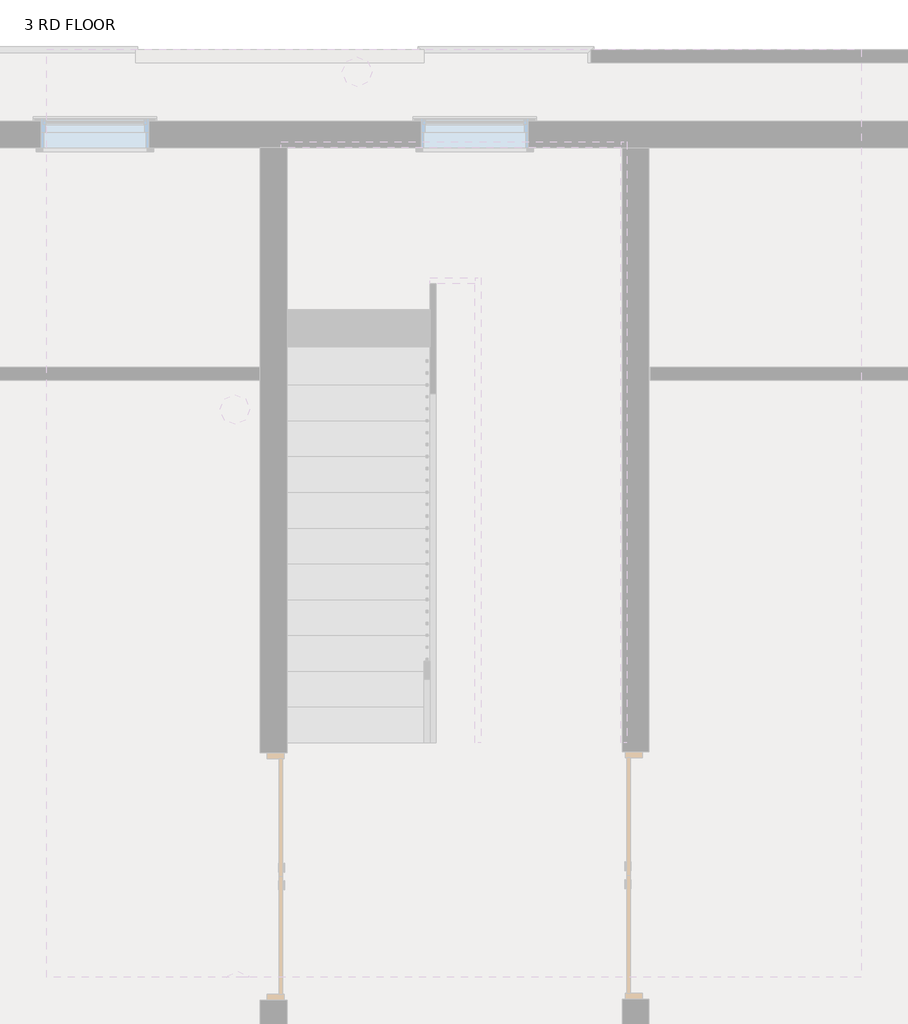
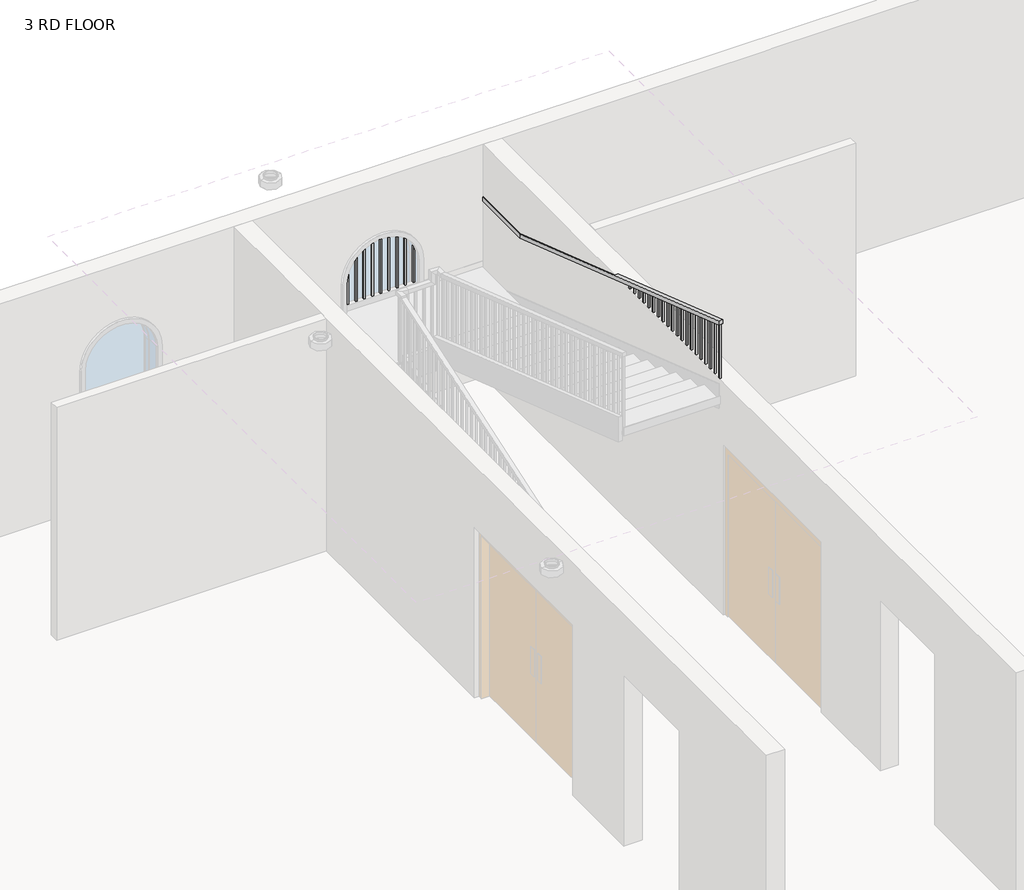
# One storey, part 5 of 7: 1 railing.
"""IFC4 building model written with IfcOpenShell, lengths in millimetres."""

from ifc_helpers import new_model, si_unit, frame, origin, place, context, project, spatial, polyline, outline, extrude, faceted_brep, element, save

model = new_model("IFC4")

# Units and contexts
model_context = context("Model", 3, world=origin())
ifc_project = project(units=[si_unit("LENGTHUNIT", "METRE", prefix="MILLI")], contexts=[model_context])

# Site, building, storey
site = spatial("IfcSite", under=ifc_project)
building = spatial("IfcBuilding", under=site)
storey = spatial("IfcBuildingStorey", under=building, Name="3 RD FLOOR", Elevation=9601.2)

# Railing
placement = place(None, origin())
element("IfcRailing", 1, ObjectType="Handrail - Rectangular", at=placement, inside=storey, context=model_context, shape_type="SolidModel", body=[
    faceted_brep([(-1899.5987998, 2564.5067329, 10619.0142857), (-1899.5987998, 2564.5067329, 10565.3699957), (-1848.7987998, 2564.5067329, 10565.3699957), (-1848.7987998, 2564.5067329, 10619.0142857), (-1899.5987998, 6526.9067329, 11963.4), (-1899.5987998, 6535.2899033, 11912.6), (-1848.7987998, 6535.2899033, 11912.6), (-1848.7987998, 6526.9067329, 11963.4), (-1899.5987998, 7682.6067329, 11912.6), (-1899.5987998, 7682.6067329, 11963.4), (1046.8012002, 7682.6067329, 11963.4), (1046.8012002, 7682.6067329, 11912.6), (-1848.7987998, 7631.8067329, 11912.6), (996.0012002, 7631.8067329, 11912.6), (-1848.7987998, 7631.8067329, 11963.4), (996.0012002, 7631.8067329, 11963.4), (1046.8012002, 6831.7067329, 11963.4), (1046.8012002, 6823.3235624, 11912.6), (996.0012002, 6823.3235624, 11912.6), (996.0012002, 6831.7067329, 11963.4), (1046.8012002, 2564.5067329, 13411.2), (996.0012002, 2564.5067329, 13411.2), (996.0012002, 2564.5067329, 13357.55571), (1046.8012002, 2564.5067329, 13357.55571)], [[[0, 1, 2, 3]], [[1, 0, 4, 5]], [[2, 1, 5, 6]], [[3, 2, 6, 7]], [[0, 3, 7, 4]], [[8, 9, 10, 11]], [[12, 8, 11, 13]], [[14, 12, 13, 15]], [[9, 14, 15, 10]], [[11, 10, 16, 17]], [[13, 11, 17, 18]], [[15, 13, 18, 19]], [[10, 15, 19, 16]], [[5, 4, 9, 8]], [[6, 5, 8, 12]], [[7, 6, 12, 14]], [[4, 7, 14, 9]], [[20, 21, 22, 23]], [[17, 16, 20, 23]], [[18, 17, 23, 22]], [[19, 18, 22, 21]], [[16, 19, 21, 20]]]),
    extrude(outline(polyline([(2586.7317329, 13350.015085), (2586.7317329, 12579.0831452), (2567.6817329, 12585.5465381), (2567.6817329, 13356.4784779), (2586.7317329, 13350.015085)])), frame((1011.8762002, 0.0, 0.0), z_axis=(1.0, 0.0, 0.0), x_axis=(0.0, 1.0, 0.0)), (0.0, 0.0, 1.0), 19.05),
    extrude(outline(polyline([(2688.3317329, 13315.5436565), (2688.3317329, 12544.6117167), (2669.2817329, 12551.0751095), (2669.2817329, 13322.0070493), (2688.3317329, 13315.5436565)])), frame((1011.8762002, 0.0, 0.0), z_axis=(1.0, 0.0, 0.0), x_axis=(0.0, 1.0, 0.0)), (0.0, 0.0, 1.0), 19.05),
    extrude(outline(polyline([(2789.9317329, 13281.0722279), (2789.9317329, 12510.1402881), (2770.8817329, 12516.603681), (2770.8817329, 13287.5356207), (2789.9317329, 13281.0722279)])), frame((1011.8762002, 0.0, 0.0), z_axis=(1.0, 0.0, 0.0), x_axis=(0.0, 1.0, 0.0)), (0.0, 0.0, 1.0), 19.05),
    extrude(outline(polyline([(2891.5317329, 13246.6007993), (2891.5317329, 12475.6688595), (2872.4817329, 12482.1322524), (2872.4817329, 13253.0641922), (2891.5317329, 13246.6007993)])), frame((1011.8762002, 0.0, 0.0), z_axis=(1.0, 0.0, 0.0), x_axis=(0.0, 1.0, 0.0)), (0.0, 0.0, 1.0), 19.05),
    extrude(outline(polyline([(2993.1317329, 13212.1293707), (2993.1317329, 12441.197431), (2974.0817329, 12447.6608238), (2974.0817329, 13218.5927636), (2993.1317329, 13212.1293707)])), frame((1011.8762002, 0.0, 0.0), z_axis=(1.0, 0.0, 0.0), x_axis=(0.0, 1.0, 0.0)), (0.0, 0.0, 1.0), 19.05),
    extrude(outline(polyline([(3094.7317329, 13177.6579422), (3094.7317329, 12406.7260024), (3075.6817329, 12413.1893952), (3075.6817329, 13184.121335), (3094.7317329, 13177.6579422)])), frame((1011.8762002, 0.0, 0.0), z_axis=(1.0, 0.0, 0.0), x_axis=(0.0, 1.0, 0.0)), (0.0, 0.0, 1.0), 19.05),
    extrude(outline(polyline([(3196.3317329, 13143.1865136), (3196.3317329, 12372.2545738), (3177.2817329, 12378.7179667), (3177.2817329, 13149.6499065), (3196.3317329, 13143.1865136)])), frame((1011.8762002, 0.0, 0.0), z_axis=(1.0, 0.0, 0.0), x_axis=(0.0, 1.0, 0.0)), (0.0, 0.0, 1.0), 19.05),
    extrude(outline(polyline([(3297.9317329, 13108.715085), (3297.9317329, 12337.7831452), (3278.8817329, 12344.2465381), (3278.8817329, 13115.1784779), (3297.9317329, 13108.715085)])), frame((1011.8762002, 0.0, 0.0), z_axis=(1.0, 0.0, 0.0), x_axis=(0.0, 1.0, 0.0)), (0.0, 0.0, 1.0), 19.05),
    extrude(outline(polyline([(3399.5317329, 13074.2436565), (3399.5317329, 12303.3117167), (3380.4817329, 12309.7751095), (3380.4817329, 13080.7070493), (3399.5317329, 13074.2436565)])), frame((1011.8762002, 0.0, 0.0), z_axis=(1.0, 0.0, 0.0), x_axis=(0.0, 1.0, 0.0)), (0.0, 0.0, 1.0), 19.05),
    extrude(outline(polyline([(3501.1317329, 13039.7722279), (3501.1317329, 12268.8402881), (3482.0817329, 12275.303681), (3482.0817329, 13046.2356207), (3501.1317329, 13039.7722279)])), frame((1011.8762002, 0.0, 0.0), z_axis=(1.0, 0.0, 0.0), x_axis=(0.0, 1.0, 0.0)), (0.0, 0.0, 1.0), 19.05),
    extrude(outline(polyline([(3602.7317329, 13005.3007993), (3602.7317329, 12234.3688595), (3583.6817329, 12240.8322524), (3583.6817329, 13011.7641922), (3602.7317329, 13005.3007993)])), frame((1011.8762002, 0.0, 0.0), z_axis=(1.0, 0.0, 0.0), x_axis=(0.0, 1.0, 0.0)), (0.0, 0.0, 1.0), 19.05),
    extrude(outline(polyline([(3704.3317329, 12970.8293707), (3704.3317329, 12199.897431), (3685.2817329, 12206.3608238), (3685.2817329, 12977.2927636), (3704.3317329, 12970.8293707)])), frame((1011.8762002, 0.0, 0.0), z_axis=(1.0, 0.0, 0.0), x_axis=(0.0, 1.0, 0.0)), (0.0, 0.0, 1.0), 19.05),
    extrude(outline(polyline([(3805.9317329, 12936.3579422), (3805.9317329, 12165.4260024), (3786.8817329, 12171.8893952), (3786.8817329, 12942.821335), (3805.9317329, 12936.3579422)])), frame((1011.8762002, 0.0, 0.0), z_axis=(1.0, 0.0, 0.0), x_axis=(0.0, 1.0, 0.0)), (0.0, 0.0, 1.0), 19.05),
    extrude(outline(polyline([(3907.5317329, 12901.8865136), (3907.5317329, 12130.9545738), (3888.4817329, 12137.4179667), (3888.4817329, 12908.3499065), (3907.5317329, 12901.8865136)])), frame((1011.8762002, 0.0, 0.0), z_axis=(1.0, 0.0, 0.0), x_axis=(0.0, 1.0, 0.0)), (0.0, 0.0, 1.0), 19.05),
    extrude(outline(polyline([(4009.1317329, 12867.415085), (4009.1317329, 12096.4831452), (3990.0817329, 12102.9465381), (3990.0817329, 12873.8784779), (4009.1317329, 12867.415085)])), frame((1011.8762002, 0.0, 0.0), z_axis=(1.0, 0.0, 0.0), x_axis=(0.0, 1.0, 0.0)), (0.0, 0.0, 1.0), 19.05),
    extrude(outline(polyline([(4110.7317329, 12832.9436565), (4110.7317329, 12062.0117167), (4091.6817329, 12068.4751095), (4091.6817329, 12839.4070493), (4110.7317329, 12832.9436565)])), frame((1011.8762002, 0.0, 0.0), z_axis=(1.0, 0.0, 0.0), x_axis=(0.0, 1.0, 0.0)), (0.0, 0.0, 1.0), 19.05),
    extrude(outline(polyline([(4212.3317329, 12798.4722279), (4212.3317329, 12027.5402881), (4193.2817329, 12034.003681), (4193.2817329, 12804.9356207), (4212.3317329, 12798.4722279)])), frame((1011.8762002, 0.0, 0.0), z_axis=(1.0, 0.0, 0.0), x_axis=(0.0, 1.0, 0.0)), (0.0, 0.0, 1.0), 19.05),
    extrude(outline(polyline([(4313.9317329, 12764.0007993), (4313.9317329, 11993.0688595), (4294.8817329, 11999.5322524), (4294.8817329, 12770.4641922), (4313.9317329, 12764.0007993)])), frame((1011.8762002, 0.0, 0.0), z_axis=(1.0, 0.0, 0.0), x_axis=(0.0, 1.0, 0.0)), (0.0, 0.0, 1.0), 19.05),
    extrude(outline(polyline([(4415.5317329, 12729.5293707), (4415.5317329, 11958.597431), (4396.4817329, 11965.0608238), (4396.4817329, 12735.9927636), (4415.5317329, 12729.5293707)])), frame((1011.8762002, 0.0, 0.0), z_axis=(1.0, 0.0, 0.0), x_axis=(0.0, 1.0, 0.0)), (0.0, 0.0, 1.0), 19.05),
    extrude(outline(polyline([(4517.1317329, 12695.0579422), (4517.1317329, 11924.1260024), (4498.0817329, 11930.5893952), (4498.0817329, 12701.521335), (4517.1317329, 12695.0579422)])), frame((1011.8762002, 0.0, 0.0), z_axis=(1.0, 0.0, 0.0), x_axis=(0.0, 1.0, 0.0)), (0.0, 0.0, 1.0), 19.05),
    extrude(outline(polyline([(4618.7317329, 12660.5865136), (4618.7317329, 11889.6545738), (4599.6817329, 11896.1179667), (4599.6817329, 12667.0499065), (4618.7317329, 12660.5865136)])), frame((1011.8762002, 0.0, 0.0), z_axis=(1.0, 0.0, 0.0), x_axis=(0.0, 1.0, 0.0)), (0.0, 0.0, 1.0), 19.05),
    extrude(outline(polyline([(4720.3317329, 12626.115085), (4720.3317329, 11855.1831452), (4701.2817329, 11861.6465381), (4701.2817329, 12632.5784779), (4720.3317329, 12626.115085)])), frame((1011.8762002, 0.0, 0.0), z_axis=(1.0, 0.0, 0.0), x_axis=(0.0, 1.0, 0.0)), (0.0, 0.0, 1.0), 19.05),
    extrude(outline(polyline([(4821.9317329, 12591.6436565), (4821.9317329, 11820.7117167), (4802.8817329, 11827.1751095), (4802.8817329, 12598.1070493), (4821.9317329, 12591.6436565)])), frame((1011.8762002, 0.0, 0.0), z_axis=(1.0, 0.0, 0.0), x_axis=(0.0, 1.0, 0.0)), (0.0, 0.0, 1.0), 19.05),
    extrude(outline(polyline([(4923.5317329, 12557.1722279), (4923.5317329, 11786.2402881), (4904.4817329, 11792.703681), (4904.4817329, 12563.6356207), (4923.5317329, 12557.1722279)])), frame((1011.8762002, 0.0, 0.0), z_axis=(1.0, 0.0, 0.0), x_axis=(0.0, 1.0, 0.0)), (0.0, 0.0, 1.0), 19.05),
    extrude(outline(polyline([(5025.1317329, 12522.7007993), (5025.1317329, 11751.7688595), (5006.0817329, 11758.2322524), (5006.0817329, 12529.1641922), (5025.1317329, 12522.7007993)])), frame((1011.8762002, 0.0, 0.0), z_axis=(1.0, 0.0, 0.0), x_axis=(0.0, 1.0, 0.0)), (0.0, 0.0, 1.0), 19.05),
    extrude(outline(polyline([(5126.7317329, 12488.2293707), (5126.7317329, 11717.297431), (5107.6817329, 11723.7608238), (5107.6817329, 12494.6927636), (5126.7317329, 12488.2293707)])), frame((1011.8762002, 0.0, 0.0), z_axis=(1.0, 0.0, 0.0), x_axis=(0.0, 1.0, 0.0)), (0.0, 0.0, 1.0), 19.05),
    extrude(outline(polyline([(5228.3317329, 12453.7579422), (5228.3317329, 11682.8260024), (5209.2817329, 11689.2893952), (5209.2817329, 12460.221335), (5228.3317329, 12453.7579422)])), frame((1011.8762002, 0.0, 0.0), z_axis=(1.0, 0.0, 0.0), x_axis=(0.0, 1.0, 0.0)), (0.0, 0.0, 1.0), 19.05),
    extrude(outline(polyline([(5329.9317329, 12419.2865136), (5329.9317329, 11648.3545738), (5310.8817329, 11654.8179667), (5310.8817329, 12425.7499065), (5329.9317329, 12419.2865136)])), frame((1011.8762002, 0.0, 0.0), z_axis=(1.0, 0.0, 0.0), x_axis=(0.0, 1.0, 0.0)), (0.0, 0.0, 1.0), 19.05),
    extrude(outline(polyline([(5431.5317329, 12384.815085), (5431.5317329, 11613.8831452), (5412.4817329, 11620.3465381), (5412.4817329, 12391.2784779), (5431.5317329, 12384.815085)])), frame((1011.8762002, 0.0, 0.0), z_axis=(1.0, 0.0, 0.0), x_axis=(0.0, 1.0, 0.0)), (0.0, 0.0, 1.0), 19.05),
    extrude(outline(polyline([(5533.1317329, 12350.3436565), (5533.1317329, 11579.4117167), (5514.0817329, 11585.8751095), (5514.0817329, 12356.8070493), (5533.1317329, 12350.3436565)])), frame((1011.8762002, 0.0, 0.0), z_axis=(1.0, 0.0, 0.0), x_axis=(0.0, 1.0, 0.0)), (0.0, 0.0, 1.0), 19.05),
    extrude(outline(polyline([(5634.7317329, 12315.8722279), (5634.7317329, 11544.9402881), (5615.6817329, 11551.403681), (5615.6817329, 12322.3356207), (5634.7317329, 12315.8722279)])), frame((1011.8762002, 0.0, 0.0), z_axis=(1.0, 0.0, 0.0), x_axis=(0.0, 1.0, 0.0)), (0.0, 0.0, 1.0), 19.05),
    extrude(outline(polyline([(5736.3317329, 12281.4007993), (5736.3317329, 11510.4688595), (5717.2817329, 11516.9322524), (5717.2817329, 12287.8641922), (5736.3317329, 12281.4007993)])), frame((1011.8762002, 0.0, 0.0), z_axis=(1.0, 0.0, 0.0), x_axis=(0.0, 1.0, 0.0)), (0.0, 0.0, 1.0), 19.05),
    extrude(outline(polyline([(5837.9317329, 12246.9293707), (5837.9317329, 11475.997431), (5818.8817329, 11482.4608238), (5818.8817329, 12253.3927636), (5837.9317329, 12246.9293707)])), frame((1011.8762002, 0.0, 0.0), z_axis=(1.0, 0.0, 0.0), x_axis=(0.0, 1.0, 0.0)), (0.0, 0.0, 1.0), 19.05),
    extrude(outline(polyline([(5939.5317329, 12212.4579422), (5939.5317329, 11441.5260024), (5920.4817329, 11447.9893952), (5920.4817329, 12218.921335), (5939.5317329, 12212.4579422)])), frame((1011.8762002, 0.0, 0.0), z_axis=(1.0, 0.0, 0.0), x_axis=(0.0, 1.0, 0.0)), (0.0, 0.0, 1.0), 19.05),
    extrude(outline(polyline([(6041.1317329, 12177.9865136), (6041.1317329, 11407.0545738), (6022.0817329, 11413.5179667), (6022.0817329, 12184.4499065), (6041.1317329, 12177.9865136)])), frame((1011.8762002, 0.0, 0.0), z_axis=(1.0, 0.0, 0.0), x_axis=(0.0, 1.0, 0.0)), (0.0, 0.0, 1.0), 19.05),
    extrude(outline(polyline([(6142.7317329, 12143.515085), (6142.7317329, 11372.5831452), (6123.6817329, 11379.0465381), (6123.6817329, 12149.9784779), (6142.7317329, 12143.515085)])), frame((1011.8762002, 0.0, 0.0), z_axis=(1.0, 0.0, 0.0), x_axis=(0.0, 1.0, 0.0)), (0.0, 0.0, 1.0), 19.05),
    extrude(outline(polyline([(6244.3317329, 12109.0436565), (6244.3317329, 11338.1117167), (6225.2817329, 11344.5751095), (6225.2817329, 12115.5070493), (6244.3317329, 12109.0436565)])), frame((1011.8762002, 0.0, 0.0), z_axis=(1.0, 0.0, 0.0), x_axis=(0.0, 1.0, 0.0)), (0.0, 0.0, 1.0), 19.05),
    extrude(outline(polyline([(6345.9317329, 12074.5722279), (6345.9317329, 11303.6402881), (6326.8817329, 11310.103681), (6326.8817329, 12081.0356207), (6345.9317329, 12074.5722279)])), frame((1011.8762002, 0.0, 0.0), z_axis=(1.0, 0.0, 0.0), x_axis=(0.0, 1.0, 0.0)), (0.0, 0.0, 1.0), 19.05),
    extrude(outline(polyline([(6447.5317329, 12040.1007993), (6447.5317329, 11269.1688595), (6428.4817329, 11275.6322524), (6428.4817329, 12046.5641922), (6447.5317329, 12040.1007993)])), frame((1011.8762002, 0.0, 0.0), z_axis=(1.0, 0.0, 0.0), x_axis=(0.0, 1.0, 0.0)), (0.0, 0.0, 1.0), 19.05),
    extrude(outline(polyline([(6549.1317329, 12005.6293707), (6549.1317329, 11234.697431), (6530.0817329, 11241.1608238), (6530.0817329, 12012.0927636), (6549.1317329, 12005.6293707)])), frame((1011.8762002, 0.0, 0.0), z_axis=(1.0, 0.0, 0.0), x_axis=(0.0, 1.0, 0.0)), (0.0, 0.0, 1.0), 19.05),
    extrude(outline(polyline([(6650.7317329, 11971.1579422), (6650.7317329, 11200.2260024), (6631.6817329, 11206.6893952), (6631.6817329, 11977.621335), (6650.7317329, 11971.1579422)])), frame((1011.8762002, 0.0, 0.0), z_axis=(1.0, 0.0, 0.0), x_axis=(0.0, 1.0, 0.0)), (0.0, 0.0, 1.0), 19.05),
    extrude(outline(polyline([(6752.3317329, 11936.6865136), (6752.3317329, 11165.7545738), (6733.2817329, 11172.2179667), (6733.2817329, 11943.1499065), (6752.3317329, 11936.6865136)])), frame((1011.8762002, 0.0, 0.0), z_axis=(1.0, 0.0, 0.0), x_axis=(0.0, 1.0, 0.0)), (0.0, 0.0, 1.0), 19.05),
    extrude(outline(polyline([(6853.9317329, 11912.6), (6853.9317329, 11131.2831452), (6834.8817329, 11137.7465381), (6834.8817329, 11912.6), (6853.9317329, 11912.6)])), frame((1011.8762002, 0.0, 0.0), z_axis=(1.0, 0.0, 0.0), x_axis=(0.0, 1.0, 0.0)), (0.0, 0.0, 1.0), 19.05),
    extrude(outline(polyline([(6955.5317329, 11912.6), (6955.5317329, 11096.8117167), (6936.4817329, 11103.2751095), (6936.4817329, 11912.6), (6955.5317329, 11912.6)])), frame((1011.8762002, 0.0, 0.0), z_axis=(1.0, 0.0, 0.0), x_axis=(0.0, 1.0, 0.0)), (0.0, 0.0, 1.0), 19.05),
    extrude(outline(polyline([(7057.1317329, 11912.6), (7057.1317329, 11062.3402881), (7038.0817329, 11068.803681), (7038.0817329, 11912.6), (7057.1317329, 11912.6)])), frame((1011.8762002, 0.0, 0.0), z_axis=(1.0, 0.0, 0.0), x_axis=(0.0, 1.0, 0.0)), (0.0, 0.0, 1.0), 19.05),
    extrude(outline(polyline([(7158.7317329, 11912.6), (7158.7317329, 11027.8688595), (7139.6817329, 11034.3322524), (7139.6817329, 11912.6), (7158.7317329, 11912.6)])), frame((1011.8762002, 0.0, 0.0), z_axis=(1.0, 0.0, 0.0), x_axis=(0.0, 1.0, 0.0)), (0.0, 0.0, 1.0), 19.05),
    extrude(outline(polyline([(7260.3317329, 11912.6), (7260.3317329, 10993.397431), (7241.2817329, 10999.8608238), (7241.2817329, 11912.6), (7260.3317329, 11912.6)])), frame((1011.8762002, 0.0, 0.0), z_axis=(1.0, 0.0, 0.0), x_axis=(0.0, 1.0, 0.0)), (0.0, 0.0, 1.0), 19.05),
    extrude(outline(polyline([(7361.9317329, 11912.6), (7361.9317329, 10958.9260024), (7342.8817329, 10965.3893952), (7342.8817329, 11912.6), (7361.9317329, 11912.6)])), frame((1011.8762002, 0.0, 0.0), z_axis=(1.0, 0.0, 0.0), x_axis=(0.0, 1.0, 0.0)), (0.0, 0.0, 1.0), 19.05),
    extrude(outline(polyline([(7463.5317329, 11912.6), (7463.5317329, 10924.4545738), (7444.4817329, 10930.9179667), (7444.4817329, 11912.6), (7463.5317329, 11912.6)])), frame((1011.8762002, 0.0, 0.0), z_axis=(1.0, 0.0, 0.0), x_axis=(0.0, 1.0, 0.0)), (0.0, 0.0, 1.0), 19.05),
    extrude(outline(polyline([(7565.1317329, 11912.6), (7565.1317329, 10889.9831452), (7546.0817329, 10896.4465381), (7546.0817329, 11912.6), (7565.1317329, 11912.6)])), frame((1011.8762002, 0.0, 0.0), z_axis=(1.0, 0.0, 0.0), x_axis=(0.0, 1.0, 0.0)), (0.0, 0.0, 1.0), 19.05),
    extrude(outline(polyline([(961.0762002, 7666.7317329), (980.1262002, 7666.7317329), (980.1262002, 7647.6817329), (961.0762002, 7647.6817329), (961.0762002, 7666.7317329)])), frame((0.0, 0.0, 11125.2), z_axis=(0.0, 0.0, 1.0), x_axis=(1.0, 0.0, 0.0)), (0.0, 0.0, 1.0), 787.4),
    extrude(outline(polyline([(859.4762002, 7666.7317329), (878.5262002, 7666.7317329), (878.5262002, 7647.6817329), (859.4762002, 7647.6817329), (859.4762002, 7666.7317329)])), frame((0.0, 0.0, 11125.2), z_axis=(0.0, 0.0, 1.0), x_axis=(1.0, 0.0, 0.0)), (0.0, 0.0, 1.0), 787.4),
    extrude(outline(polyline([(757.8762002, 7666.7317329), (776.9262002, 7666.7317329), (776.9262002, 7647.6817329), (757.8762002, 7647.6817329), (757.8762002, 7666.7317329)])), frame((0.0, 0.0, 11125.2), z_axis=(0.0, 0.0, 1.0), x_axis=(1.0, 0.0, 0.0)), (0.0, 0.0, 1.0), 787.4),
    extrude(outline(polyline([(656.2762002, 7666.7317329), (675.3262002, 7666.7317329), (675.3262002, 7647.6817329), (656.2762002, 7647.6817329), (656.2762002, 7666.7317329)])), frame((0.0, 0.0, 11125.2), z_axis=(0.0, 0.0, 1.0), x_axis=(1.0, 0.0, 0.0)), (0.0, 0.0, 1.0), 787.4),
    extrude(outline(polyline([(554.6762002, 7666.7317329), (573.7262002, 7666.7317329), (573.7262002, 7647.6817329), (554.6762002, 7647.6817329), (554.6762002, 7666.7317329)])), frame((0.0, 0.0, 11125.2), z_axis=(0.0, 0.0, 1.0), x_axis=(1.0, 0.0, 0.0)), (0.0, 0.0, 1.0), 787.4),
    extrude(outline(polyline([(453.0762002, 7666.7317329), (472.1262002, 7666.7317329), (472.1262002, 7647.6817329), (453.0762002, 7647.6817329), (453.0762002, 7666.7317329)])), frame((0.0, 0.0, 11125.2), z_axis=(0.0, 0.0, 1.0), x_axis=(1.0, 0.0, 0.0)), (0.0, 0.0, 1.0), 787.4),
    extrude(outline(polyline([(351.4762002, 7666.7317329), (370.5262002, 7666.7317329), (370.5262002, 7647.6817329), (351.4762002, 7647.6817329), (351.4762002, 7666.7317329)])), frame((0.0, 0.0, 11125.2), z_axis=(0.0, 0.0, 1.0), x_axis=(1.0, 0.0, 0.0)), (0.0, 0.0, 1.0), 787.4),
    extrude(outline(polyline([(249.8762002, 7666.7317329), (268.9262002, 7666.7317329), (268.9262002, 7647.6817329), (249.8762002, 7647.6817329), (249.8762002, 7666.7317329)])), frame((0.0, 0.0, 11125.2), z_axis=(0.0, 0.0, 1.0), x_axis=(1.0, 0.0, 0.0)), (0.0, 0.0, 1.0), 787.4),
    extrude(outline(polyline([(148.2762002, 7666.7317329), (167.3262002, 7666.7317329), (167.3262002, 7647.6817329), (148.2762002, 7647.6817329), (148.2762002, 7666.7317329)])), frame((0.0, 0.0, 11125.2), z_axis=(0.0, 0.0, 1.0), x_axis=(1.0, 0.0, 0.0)), (0.0, 0.0, 1.0), 787.4),
    extrude(outline(polyline([(46.6762002, 7666.7317329), (65.7262002, 7666.7317329), (65.7262002, 7647.6817329), (46.6762002, 7647.6817329), (46.6762002, 7666.7317329)])), frame((0.0, 0.0, 11125.2), z_axis=(0.0, 0.0, 1.0), x_axis=(1.0, 0.0, 0.0)), (0.0, 0.0, 1.0), 787.4),
    extrude(outline(polyline([(-54.9237998, 7666.7317329), (-35.8737998, 7666.7317329), (-35.8737998, 7647.6817329), (-54.9237998, 7647.6817329), (-54.9237998, 7666.7317329)])), frame((0.0, 0.0, 11125.2), z_axis=(0.0, 0.0, 1.0), x_axis=(1.0, 0.0, 0.0)), (0.0, 0.0, 1.0), 787.4),
    extrude(outline(polyline([(-156.5237998, 7666.7317329), (-137.4737998, 7666.7317329), (-137.4737998, 7647.6817329), (-156.5237998, 7647.6817329), (-156.5237998, 7666.7317329)])), frame((0.0, 0.0, 11125.2), z_axis=(0.0, 0.0, 1.0), x_axis=(1.0, 0.0, 0.0)), (0.0, 0.0, 1.0), 787.4),
    extrude(outline(polyline([(-258.1237998, 7666.7317329), (-239.0737998, 7666.7317329), (-239.0737998, 7647.6817329), (-258.1237998, 7647.6817329), (-258.1237998, 7666.7317329)])), frame((0.0, 0.0, 11125.2), z_axis=(0.0, 0.0, 1.0), x_axis=(1.0, 0.0, 0.0)), (0.0, 0.0, 1.0), 787.4),
    extrude(outline(polyline([(-359.7237998, 7666.7317329), (-340.6737998, 7666.7317329), (-340.6737998, 7647.6817329), (-359.7237998, 7647.6817329), (-359.7237998, 7666.7317329)])), frame((0.0, 0.0, 11125.2), z_axis=(0.0, 0.0, 1.0), x_axis=(1.0, 0.0, 0.0)), (0.0, 0.0, 1.0), 787.4),
    extrude(outline(polyline([(-461.3237998, 7666.7317329), (-442.2737998, 7666.7317329), (-442.2737998, 7647.6817329), (-461.3237998, 7647.6817329), (-461.3237998, 7666.7317329)])), frame((0.0, 0.0, 11125.2), z_axis=(0.0, 0.0, 1.0), x_axis=(1.0, 0.0, 0.0)), (0.0, 0.0, 1.0), 787.4),
    extrude(outline(polyline([(-562.9237998, 7666.7317329), (-543.8737998, 7666.7317329), (-543.8737998, 7647.6817329), (-562.9237998, 7647.6817329), (-562.9237998, 7666.7317329)])), frame((0.0, 0.0, 11125.2), z_axis=(0.0, 0.0, 1.0), x_axis=(1.0, 0.0, 0.0)), (0.0, 0.0, 1.0), 787.4),
    extrude(outline(polyline([(-664.5237998, 7666.7317329), (-645.4737998, 7666.7317329), (-645.4737998, 7647.6817329), (-664.5237998, 7647.6817329), (-664.5237998, 7666.7317329)])), frame((0.0, 0.0, 11125.2), z_axis=(0.0, 0.0, 1.0), x_axis=(1.0, 0.0, 0.0)), (0.0, 0.0, 1.0), 787.4),
    extrude(outline(polyline([(-766.1237998, 7666.7317329), (-747.0737998, 7666.7317329), (-747.0737998, 7647.6817329), (-766.1237998, 7647.6817329), (-766.1237998, 7666.7317329)])), frame((0.0, 0.0, 11125.2), z_axis=(0.0, 0.0, 1.0), x_axis=(1.0, 0.0, 0.0)), (0.0, 0.0, 1.0), 787.4),
    extrude(outline(polyline([(-867.7237998, 7666.7317329), (-848.6737998, 7666.7317329), (-848.6737998, 7647.6817329), (-867.7237998, 7647.6817329), (-867.7237998, 7666.7317329)])), frame((0.0, 0.0, 11125.2), z_axis=(0.0, 0.0, 1.0), x_axis=(1.0, 0.0, 0.0)), (0.0, 0.0, 1.0), 787.4),
    extrude(outline(polyline([(-969.3237998, 7666.7317329), (-950.2737998, 7666.7317329), (-950.2737998, 7647.6817329), (-969.3237998, 7647.6817329), (-969.3237998, 7666.7317329)])), frame((0.0, 0.0, 11125.2), z_axis=(0.0, 0.0, 1.0), x_axis=(1.0, 0.0, 0.0)), (0.0, 0.0, 1.0), 787.4),
    extrude(outline(polyline([(-1070.9237998, 7666.7317329), (-1051.8737998, 7666.7317329), (-1051.8737998, 7647.6817329), (-1070.9237998, 7647.6817329), (-1070.9237998, 7666.7317329)])), frame((0.0, 0.0, 11125.2), z_axis=(0.0, 0.0, 1.0), x_axis=(1.0, 0.0, 0.0)), (0.0, 0.0, 1.0), 787.4),
    extrude(outline(polyline([(-1172.5237998, 7666.7317329), (-1153.4737998, 7666.7317329), (-1153.4737998, 7647.6817329), (-1172.5237998, 7647.6817329), (-1172.5237998, 7666.7317329)])), frame((0.0, 0.0, 11125.2), z_axis=(0.0, 0.0, 1.0), x_axis=(1.0, 0.0, 0.0)), (0.0, 0.0, 1.0), 787.4),
    extrude(outline(polyline([(-1274.1237998, 7666.7317329), (-1255.0737998, 7666.7317329), (-1255.0737998, 7647.6817329), (-1274.1237998, 7647.6817329), (-1274.1237998, 7666.7317329)])), frame((0.0, 0.0, 11125.2), z_axis=(0.0, 0.0, 1.0), x_axis=(1.0, 0.0, 0.0)), (0.0, 0.0, 1.0), 787.4),
    extrude(outline(polyline([(-1375.7237998, 7666.7317329), (-1356.6737998, 7666.7317329), (-1356.6737998, 7647.6817329), (-1375.7237998, 7647.6817329), (-1375.7237998, 7666.7317329)])), frame((0.0, 0.0, 11125.2), z_axis=(0.0, 0.0, 1.0), x_axis=(1.0, 0.0, 0.0)), (0.0, 0.0, 1.0), 787.4),
    extrude(outline(polyline([(-1477.3237998, 7666.7317329), (-1458.2737998, 7666.7317329), (-1458.2737998, 7647.6817329), (-1477.3237998, 7647.6817329), (-1477.3237998, 7666.7317329)])), frame((0.0, 0.0, 11125.2), z_axis=(0.0, 0.0, 1.0), x_axis=(1.0, 0.0, 0.0)), (0.0, 0.0, 1.0), 787.4),
    extrude(outline(polyline([(-1578.9237998, 7666.7317329), (-1559.8737998, 7666.7317329), (-1559.8737998, 7647.6817329), (-1578.9237998, 7647.6817329), (-1578.9237998, 7666.7317329)])), frame((0.0, 0.0, 11125.2), z_axis=(0.0, 0.0, 1.0), x_axis=(1.0, 0.0, 0.0)), (0.0, 0.0, 1.0), 787.4),
    extrude(outline(polyline([(-1680.5237998, 7666.7317329), (-1661.4737998, 7666.7317329), (-1661.4737998, 7647.6817329), (-1680.5237998, 7647.6817329), (-1680.5237998, 7666.7317329)])), frame((0.0, 0.0, 11125.2), z_axis=(0.0, 0.0, 1.0), x_axis=(1.0, 0.0, 0.0)), (0.0, 0.0, 1.0), 787.4),
    extrude(outline(polyline([(-1782.1237998, 7666.7317329), (-1763.0737998, 7666.7317329), (-1763.0737998, 7647.6817329), (-1782.1237998, 7647.6817329), (-1782.1237998, 7666.7317329)])), frame((0.0, 0.0, 11125.2), z_axis=(0.0, 0.0, 1.0), x_axis=(1.0, 0.0, 0.0)), (0.0, 0.0, 1.0), 787.4),
    extrude(outline(polyline([(-1883.7237998, 7634.9817329), (-1883.7237998, 7654.0317329), (-1864.6737998, 7654.0317329), (-1864.6737998, 7634.9817329), (-1883.7237998, 7634.9817329)])), frame((0.0, 0.0, 11428.1857143), z_axis=(0.0, 0.0, 1.0), x_axis=(1.0, 0.0, 0.0)), (0.0, 0.0, 1.0), 484.4142857),
    extrude(outline(polyline([(-1883.7237998, 7533.3817329), (-1883.7237998, 7552.4317329), (-1864.6737998, 7552.4317329), (-1864.6737998, 7533.3817329), (-1883.7237998, 7533.3817329)])), frame((0.0, 0.0, 11393.7142857), z_axis=(0.0, 0.0, 1.0), x_axis=(1.0, 0.0, 0.0)), (0.0, 0.0, 1.0), 518.8857143),
    extrude(outline(polyline([(-1883.7237998, 7431.7817329), (-1883.7237998, 7450.8317329), (-1864.6737998, 7450.8317329), (-1864.6737998, 7431.7817329), (-1883.7237998, 7431.7817329)])), frame((0.0, 0.0, 11359.2428571), z_axis=(0.0, 0.0, 1.0), x_axis=(1.0, 0.0, 0.0)), (0.0, 0.0, 1.0), 553.3571429),
    extrude(outline(polyline([(-1883.7237998, 7330.1817329), (-1883.7237998, 7349.2317329), (-1864.6737998, 7349.2317329), (-1864.6737998, 7330.1817329), (-1883.7237998, 7330.1817329)])), frame((0.0, 0.0, 11324.7714286), z_axis=(0.0, 0.0, 1.0), x_axis=(1.0, 0.0, 0.0)), (0.0, 0.0, 1.0), 587.8285714),
    extrude(outline(polyline([(-1883.7237998, 7228.5817329), (-1883.7237998, 7247.6317329), (-1864.6737998, 7247.6317329), (-1864.6737998, 7228.5817329), (-1883.7237998, 7228.5817329)])), frame((0.0, 0.0, 11290.3), z_axis=(0.0, 0.0, 1.0), x_axis=(1.0, 0.0, 0.0)), (0.0, 0.0, 1.0), 622.3),
    extrude(outline(polyline([(-1883.7237998, 7126.9817329), (-1883.7237998, 7146.0317329), (-1864.6737998, 7146.0317329), (-1864.6737998, 7126.9817329), (-1883.7237998, 7126.9817329)])), frame((0.0, 0.0, 11255.8285714), z_axis=(0.0, 0.0, 1.0), x_axis=(1.0, 0.0, 0.0)), (0.0, 0.0, 1.0), 656.7714286),
    extrude(outline(polyline([(-1883.7237998, 7025.3817329), (-1883.7237998, 7044.4317329), (-1864.6737998, 7044.4317329), (-1864.6737998, 7025.3817329), (-1883.7237998, 7025.3817329)])), frame((0.0, 0.0, 11125.2), z_axis=(0.0, 0.0, 1.0), x_axis=(1.0, 0.0, 0.0)), (0.0, 0.0, 1.0), 787.4),
    extrude(outline(polyline([(-1883.7237998, 6923.7817329), (-1883.7237998, 6942.8317329), (-1864.6737998, 6942.8317329), (-1864.6737998, 6923.7817329), (-1883.7237998, 6923.7817329)])), frame((0.0, 0.0, 11125.2), z_axis=(0.0, 0.0, 1.0), x_axis=(1.0, 0.0, 0.0)), (0.0, 0.0, 1.0), 787.4),
    extrude(outline(polyline([(-1883.7237998, 6822.1817329), (-1883.7237998, 6841.2317329), (-1864.6737998, 6841.2317329), (-1864.6737998, 6822.1817329), (-1883.7237998, 6822.1817329)])), frame((0.0, 0.0, 11125.2), z_axis=(0.0, 0.0, 1.0), x_axis=(1.0, 0.0, 0.0)), (0.0, 0.0, 1.0), 787.4),
    extrude(outline(polyline([(-1883.7237998, 6720.5817329), (-1883.7237998, 6739.6317329), (-1864.6737998, 6739.6317329), (-1864.6737998, 6720.5817329), (-1883.7237998, 6720.5817329)])), frame((0.0, 0.0, 11125.2), z_axis=(0.0, 0.0, 1.0), x_axis=(1.0, 0.0, 0.0)), (0.0, 0.0, 1.0), 787.4),
    extrude(outline(polyline([(-1883.7237998, 6618.9817329), (-1883.7237998, 6638.0317329), (-1864.6737998, 6638.0317329), (-1864.6737998, 6618.9817329), (-1883.7237998, 6618.9817329)])), frame((0.0, 0.0, 11125.2), z_axis=(0.0, 0.0, 1.0), x_axis=(1.0, 0.0, 0.0)), (0.0, 0.0, 1.0), 787.4),
    extrude(outline(polyline([(6536.4317329, 11912.9874065), (6536.4317329, 11125.2), (6517.3817329, 11125.2), (6517.3817329, 11906.5240136), (6536.4317329, 11912.9874065)])), frame((-1883.7237998, 0.0, 0.0), z_axis=(1.0, 0.0, 0.0), x_axis=(0.0, 1.0, 0.0)), (0.0, 0.0, 1.0), 19.05),
    extrude(outline(polyline([(6434.8317329, 11878.5159779), (6434.8317329, 11107.5840381), (6415.7817329, 11101.1206452), (6415.7817329, 11872.052585), (6434.8317329, 11878.5159779)])), frame((-1883.7237998, 0.0, 0.0), z_axis=(1.0, 0.0, 0.0), x_axis=(0.0, 1.0, 0.0)), (0.0, 0.0, 1.0), 19.05),
    extrude(outline(polyline([(6333.2317329, 11844.0445493), (6333.2317329, 11073.1126095), (6314.1817329, 11066.6492167), (6314.1817329, 11837.5811565), (6333.2317329, 11844.0445493)])), frame((-1883.7237998, 0.0, 0.0), z_axis=(1.0, 0.0, 0.0), x_axis=(0.0, 1.0, 0.0)), (0.0, 0.0, 1.0), 19.05),
    extrude(outline(polyline([(6231.6317329, 11809.5731207), (6231.6317329, 11038.641181), (6212.5817329, 11032.1777881), (6212.5817329, 11803.1097279), (6231.6317329, 11809.5731207)])), frame((-1883.7237998, 0.0, 0.0), z_axis=(1.0, 0.0, 0.0), x_axis=(0.0, 1.0, 0.0)), (0.0, 0.0, 1.0), 19.05),
    extrude(outline(polyline([(6130.0317329, 11775.1016922), (6130.0317329, 11004.1697524), (6110.9817329, 10997.7063595), (6110.9817329, 11768.6382993), (6130.0317329, 11775.1016922)])), frame((-1883.7237998, 0.0, 0.0), z_axis=(1.0, 0.0, 0.0), x_axis=(0.0, 1.0, 0.0)), (0.0, 0.0, 1.0), 19.05),
    extrude(outline(polyline([(6028.4317329, 11740.6302636), (6028.4317329, 10969.6983238), (6009.3817329, 10963.234931), (6009.3817329, 11734.1668707), (6028.4317329, 11740.6302636)])), frame((-1883.7237998, 0.0, 0.0), z_axis=(1.0, 0.0, 0.0), x_axis=(0.0, 1.0, 0.0)), (0.0, 0.0, 1.0), 19.05),
    extrude(outline(polyline([(5926.8317329, 11706.158835), (5926.8317329, 10935.2268952), (5907.7817329, 10928.7635024), (5907.7817329, 11699.6954422), (5926.8317329, 11706.158835)])), frame((-1883.7237998, 0.0, 0.0), z_axis=(1.0, 0.0, 0.0), x_axis=(0.0, 1.0, 0.0)), (0.0, 0.0, 1.0), 19.05),
    extrude(outline(polyline([(5825.2317329, 11671.6874065), (5825.2317329, 10900.7554667), (5806.1817329, 10894.2920738), (5806.1817329, 11665.2240136), (5825.2317329, 11671.6874065)])), frame((-1883.7237998, 0.0, 0.0), z_axis=(1.0, 0.0, 0.0), x_axis=(0.0, 1.0, 0.0)), (0.0, 0.0, 1.0), 19.05),
    extrude(outline(polyline([(5723.6317329, 11637.2159779), (5723.6317329, 10866.2840381), (5704.5817329, 10859.8206452), (5704.5817329, 11630.752585), (5723.6317329, 11637.2159779)])), frame((-1883.7237998, 0.0, 0.0), z_axis=(1.0, 0.0, 0.0), x_axis=(0.0, 1.0, 0.0)), (0.0, 0.0, 1.0), 19.05),
    extrude(outline(polyline([(5622.0317329, 11602.7445493), (5622.0317329, 10831.8126095), (5602.9817329, 10825.3492167), (5602.9817329, 11596.2811565), (5622.0317329, 11602.7445493)])), frame((-1883.7237998, 0.0, 0.0), z_axis=(1.0, 0.0, 0.0), x_axis=(0.0, 1.0, 0.0)), (0.0, 0.0, 1.0), 19.05),
    extrude(outline(polyline([(5520.4317329, 11568.2731207), (5520.4317329, 10797.341181), (5501.3817329, 10790.8777881), (5501.3817329, 11561.8097279), (5520.4317329, 11568.2731207)])), frame((-1883.7237998, 0.0, 0.0), z_axis=(1.0, 0.0, 0.0), x_axis=(0.0, 1.0, 0.0)), (0.0, 0.0, 1.0), 19.05),
    extrude(outline(polyline([(5418.8317329, 11533.8016922), (5418.8317329, 10762.8697524), (5399.7817329, 10756.4063595), (5399.7817329, 11527.3382993), (5418.8317329, 11533.8016922)])), frame((-1883.7237998, 0.0, 0.0), z_axis=(1.0, 0.0, 0.0), x_axis=(0.0, 1.0, 0.0)), (0.0, 0.0, 1.0), 19.05),
    extrude(outline(polyline([(5317.2317329, 11499.3302636), (5317.2317329, 10728.3983238), (5298.1817329, 10721.934931), (5298.1817329, 11492.8668707), (5317.2317329, 11499.3302636)])), frame((-1883.7237998, 0.0, 0.0), z_axis=(1.0, 0.0, 0.0), x_axis=(0.0, 1.0, 0.0)), (0.0, 0.0, 1.0), 19.05),
    extrude(outline(polyline([(5215.6317329, 11464.858835), (5215.6317329, 10693.9268952), (5196.5817329, 10687.4635024), (5196.5817329, 11458.3954422), (5215.6317329, 11464.858835)])), frame((-1883.7237998, 0.0, 0.0), z_axis=(1.0, 0.0, 0.0), x_axis=(0.0, 1.0, 0.0)), (0.0, 0.0, 1.0), 19.05),
    extrude(outline(polyline([(5114.0317329, 11430.3874065), (5114.0317329, 10659.4554667), (5094.9817329, 10652.9920738), (5094.9817329, 11423.9240136), (5114.0317329, 11430.3874065)])), frame((-1883.7237998, 0.0, 0.0), z_axis=(1.0, 0.0, 0.0), x_axis=(0.0, 1.0, 0.0)), (0.0, 0.0, 1.0), 19.05),
    extrude(outline(polyline([(5012.4317329, 11395.9159779), (5012.4317329, 10624.9840381), (4993.3817329, 10618.5206452), (4993.3817329, 11389.452585), (5012.4317329, 11395.9159779)])), frame((-1883.7237998, 0.0, 0.0), z_axis=(1.0, 0.0, 0.0), x_axis=(0.0, 1.0, 0.0)), (0.0, 0.0, 1.0), 19.05),
    extrude(outline(polyline([(4910.8317329, 11361.4445493), (4910.8317329, 10590.5126095), (4891.7817329, 10584.0492167), (4891.7817329, 11354.9811565), (4910.8317329, 11361.4445493)])), frame((-1883.7237998, 0.0, 0.0), z_axis=(1.0, 0.0, 0.0), x_axis=(0.0, 1.0, 0.0)), (0.0, 0.0, 1.0), 19.05),
    extrude(outline(polyline([(4809.2317329, 11326.9731207), (4809.2317329, 10556.041181), (4790.1817329, 10549.5777881), (4790.1817329, 11320.5097279), (4809.2317329, 11326.9731207)])), frame((-1883.7237998, 0.0, 0.0), z_axis=(1.0, 0.0, 0.0), x_axis=(0.0, 1.0, 0.0)), (0.0, 0.0, 1.0), 19.05),
    extrude(outline(polyline([(4707.6317329, 11292.5016922), (4707.6317329, 10521.5697524), (4688.5817329, 10515.1063595), (4688.5817329, 11286.0382993), (4707.6317329, 11292.5016922)])), frame((-1883.7237998, 0.0, 0.0), z_axis=(1.0, 0.0, 0.0), x_axis=(0.0, 1.0, 0.0)), (0.0, 0.0, 1.0), 19.05),
    extrude(outline(polyline([(4606.0317329, 11258.0302636), (4606.0317329, 10487.0983238), (4586.9817329, 10480.634931), (4586.9817329, 11251.5668707), (4606.0317329, 11258.0302636)])), frame((-1883.7237998, 0.0, 0.0), z_axis=(1.0, 0.0, 0.0), x_axis=(0.0, 1.0, 0.0)), (0.0, 0.0, 1.0), 19.05),
    extrude(outline(polyline([(4504.4317329, 11223.558835), (4504.4317329, 10452.6268952), (4485.3817329, 10446.1635024), (4485.3817329, 11217.0954422), (4504.4317329, 11223.558835)])), frame((-1883.7237998, 0.0, 0.0), z_axis=(1.0, 0.0, 0.0), x_axis=(0.0, 1.0, 0.0)), (0.0, 0.0, 1.0), 19.05),
    extrude(outline(polyline([(4402.8317329, 11189.0874065), (4402.8317329, 10418.1554667), (4383.7817329, 10411.6920738), (4383.7817329, 11182.6240136), (4402.8317329, 11189.0874065)])), frame((-1883.7237998, 0.0, 0.0), z_axis=(1.0, 0.0, 0.0), x_axis=(0.0, 1.0, 0.0)), (0.0, 0.0, 1.0), 19.05),
    extrude(outline(polyline([(4301.2317329, 11154.6159779), (4301.2317329, 10383.6840381), (4282.1817329, 10377.2206452), (4282.1817329, 11148.152585), (4301.2317329, 11154.6159779)])), frame((-1883.7237998, 0.0, 0.0), z_axis=(1.0, 0.0, 0.0), x_axis=(0.0, 1.0, 0.0)), (0.0, 0.0, 1.0), 19.05),
    extrude(outline(polyline([(4199.6317329, 11120.1445493), (4199.6317329, 10349.2126095), (4180.5817329, 10342.7492167), (4180.5817329, 11113.6811565), (4199.6317329, 11120.1445493)])), frame((-1883.7237998, 0.0, 0.0), z_axis=(1.0, 0.0, 0.0), x_axis=(0.0, 1.0, 0.0)), (0.0, 0.0, 1.0), 19.05),
    extrude(outline(polyline([(4098.0317329, 11085.6731207), (4098.0317329, 10314.741181), (4078.9817329, 10308.2777881), (4078.9817329, 11079.2097279), (4098.0317329, 11085.6731207)])), frame((-1883.7237998, 0.0, 0.0), z_axis=(1.0, 0.0, 0.0), x_axis=(0.0, 1.0, 0.0)), (0.0, 0.0, 1.0), 19.05),
    extrude(outline(polyline([(3996.4317329, 11051.2016922), (3996.4317329, 10280.2697524), (3977.3817329, 10273.8063595), (3977.3817329, 11044.7382993), (3996.4317329, 11051.2016922)])), frame((-1883.7237998, 0.0, 0.0), z_axis=(1.0, 0.0, 0.0), x_axis=(0.0, 1.0, 0.0)), (0.0, 0.0, 1.0), 19.05),
    extrude(outline(polyline([(3894.8317329, 11016.7302636), (3894.8317329, 10245.7983238), (3875.7817329, 10239.334931), (3875.7817329, 11010.2668707), (3894.8317329, 11016.7302636)])), frame((-1883.7237998, 0.0, 0.0), z_axis=(1.0, 0.0, 0.0), x_axis=(0.0, 1.0, 0.0)), (0.0, 0.0, 1.0), 19.05),
    extrude(outline(polyline([(3793.2317329, 10982.258835), (3793.2317329, 10211.3268952), (3774.1817329, 10204.8635024), (3774.1817329, 10975.7954422), (3793.2317329, 10982.258835)])), frame((-1883.7237998, 0.0, 0.0), z_axis=(1.0, 0.0, 0.0), x_axis=(0.0, 1.0, 0.0)), (0.0, 0.0, 1.0), 19.05),
    extrude(outline(polyline([(3691.6317329, 10947.7874065), (3691.6317329, 10176.8554667), (3672.5817329, 10170.3920738), (3672.5817329, 10941.3240136), (3691.6317329, 10947.7874065)])), frame((-1883.7237998, 0.0, 0.0), z_axis=(1.0, 0.0, 0.0), x_axis=(0.0, 1.0, 0.0)), (0.0, 0.0, 1.0), 19.05),
    extrude(outline(polyline([(3590.0317329, 10913.3159779), (3590.0317329, 10142.3840381), (3570.9817329, 10135.9206452), (3570.9817329, 10906.852585), (3590.0317329, 10913.3159779)])), frame((-1883.7237998, 0.0, 0.0), z_axis=(1.0, 0.0, 0.0), x_axis=(0.0, 1.0, 0.0)), (0.0, 0.0, 1.0), 19.05),
    extrude(outline(polyline([(3488.4317329, 10878.8445493), (3488.4317329, 10107.9126095), (3469.3817329, 10101.4492167), (3469.3817329, 10872.3811565), (3488.4317329, 10878.8445493)])), frame((-1883.7237998, 0.0, 0.0), z_axis=(1.0, 0.0, 0.0), x_axis=(0.0, 1.0, 0.0)), (0.0, 0.0, 1.0), 19.05),
    extrude(outline(polyline([(3386.8317329, 10844.3731207), (3386.8317329, 10073.441181), (3367.7817329, 10066.9777881), (3367.7817329, 10837.9097279), (3386.8317329, 10844.3731207)])), frame((-1883.7237998, 0.0, 0.0), z_axis=(1.0, 0.0, 0.0), x_axis=(0.0, 1.0, 0.0)), (0.0, 0.0, 1.0), 19.05),
    extrude(outline(polyline([(3285.2317329, 10809.9016922), (3285.2317329, 10038.9697524), (3266.1817329, 10032.5063595), (3266.1817329, 10803.4382993), (3285.2317329, 10809.9016922)])), frame((-1883.7237998, 0.0, 0.0), z_axis=(1.0, 0.0, 0.0), x_axis=(0.0, 1.0, 0.0)), (0.0, 0.0, 1.0), 19.05),
    extrude(outline(polyline([(3183.6317329, 10775.4302636), (3183.6317329, 10004.4983238), (3164.5817329, 9998.034931), (3164.5817329, 10768.9668707), (3183.6317329, 10775.4302636)])), frame((-1883.7237998, 0.0, 0.0), z_axis=(1.0, 0.0, 0.0), x_axis=(0.0, 1.0, 0.0)), (0.0, 0.0, 1.0), 19.05),
    extrude(outline(polyline([(3082.0317329, 10740.958835), (3082.0317329, 9970.0268952), (3062.9817329, 9963.5635024), (3062.9817329, 10734.4954422), (3082.0317329, 10740.958835)])), frame((-1883.7237998, 0.0, 0.0), z_axis=(1.0, 0.0, 0.0), x_axis=(0.0, 1.0, 0.0)), (0.0, 0.0, 1.0), 19.05),
    extrude(outline(polyline([(2980.4317329, 10706.4874065), (2980.4317329, 9935.5554667), (2961.3817329, 9929.0920738), (2961.3817329, 10700.0240136), (2980.4317329, 10706.4874065)])), frame((-1883.7237998, 0.0, 0.0), z_axis=(1.0, 0.0, 0.0), x_axis=(0.0, 1.0, 0.0)), (0.0, 0.0, 1.0), 19.05),
    extrude(outline(polyline([(2878.8317329, 10672.0159779), (2878.8317329, 9901.0840381), (2859.7817329, 9894.6206452), (2859.7817329, 10665.552585), (2878.8317329, 10672.0159779)])), frame((-1883.7237998, 0.0, 0.0), z_axis=(1.0, 0.0, 0.0), x_axis=(0.0, 1.0, 0.0)), (0.0, 0.0, 1.0), 19.05),
    extrude(outline(polyline([(2777.2317329, 10637.5445493), (2777.2317329, 9866.6126095), (2758.1817329, 9860.1492167), (2758.1817329, 10631.0811565), (2777.2317329, 10637.5445493)])), frame((-1883.7237998, 0.0, 0.0), z_axis=(1.0, 0.0, 0.0), x_axis=(0.0, 1.0, 0.0)), (0.0, 0.0, 1.0), 19.05),
    extrude(outline(polyline([(2675.6317329, 10603.0731207), (2675.6317329, 9832.141181), (2656.5817329, 9825.6777881), (2656.5817329, 10596.6097279), (2675.6317329, 10603.0731207)])), frame((-1883.7237998, 0.0, 0.0), z_axis=(1.0, 0.0, 0.0), x_axis=(0.0, 1.0, 0.0)), (0.0, 0.0, 1.0), 19.05),
    extrude(outline(polyline([(1011.8762002, 7666.7317329), (1030.9262002, 7666.7317329), (1030.9262002, 7647.6817329), (1011.8762002, 7647.6817329), (1011.8762002, 7666.7317329)])), frame((0.0, 0.0, 11049.0), z_axis=(0.0, 0.0, 1.0), x_axis=(1.0, 0.0, 0.0)), (0.0, 0.0, 1.0), 863.6),
    extrude(outline(polyline([(-1883.7237998, 7647.6817329), (-1883.7237998, 7666.7317329), (-1864.6737998, 7666.7317329), (-1864.6737998, 7647.6817329), (-1883.7237998, 7647.6817329)])), frame((0.0, 0.0, 11432.4946428), z_axis=(0.0, 0.0, 1.0), x_axis=(1.0, 0.0, 0.0)), (0.0, 0.0, 1.0), 480.1053572),
    extrude(outline(polyline([(2583.5567329, 13351.0923172), (2583.5567329, 12580.1603774), (2564.5067329, 12586.6237702), (2564.5067329, 13357.55571), (2583.5567329, 13351.0923172)])), frame((1011.8762002, 0.0, 0.0), z_axis=(1.0, 0.0, 0.0), x_axis=(0.0, 1.0, 0.0)), (0.0, 0.0, 1.0), 19.05),
    extrude(outline(polyline([(2583.5567329, 10571.8333886), (2583.5567329, 9800.9014488), (2564.5067329, 9794.438056), (2564.5067329, 10565.3699957), (2583.5567329, 10571.8333886)])), frame((-1883.7237998, 0.0, 0.0), z_axis=(1.0, 0.0, 0.0), x_axis=(0.0, 1.0, 0.0)), (0.0, 0.0, 1.0), 19.05),
])

save(model, "model.ifc")

# Revit data of these elements
# Type "Handrail - Rectangular"
#   Assembly Code = "C2010400"
#   built-in parameter 1008612 = 0.0416667 (stored number, unit not read)
#   built-in parameter 1008611 = 0.0416667 (stored number, unit not read)
#   built-in parameter 1008609 = 0.333333 (stored number, unit not read)
#   built-in parameter 1008604 = 0.166667 (stored number, unit not read)
#   built-in parameter 1008603 = 0.166667 (stored number, unit not read)
#   Railing Height = 3' - 0"
#   built-in parameter 1008630 = 2
#   built-in parameter 1008610 = 2
#   built-in parameter 1008618 = Baluster - Square : 3/4"
# Element 1 (IfcRailing, "Handrail - Rectangular")
#   Phase Created = New Construction
